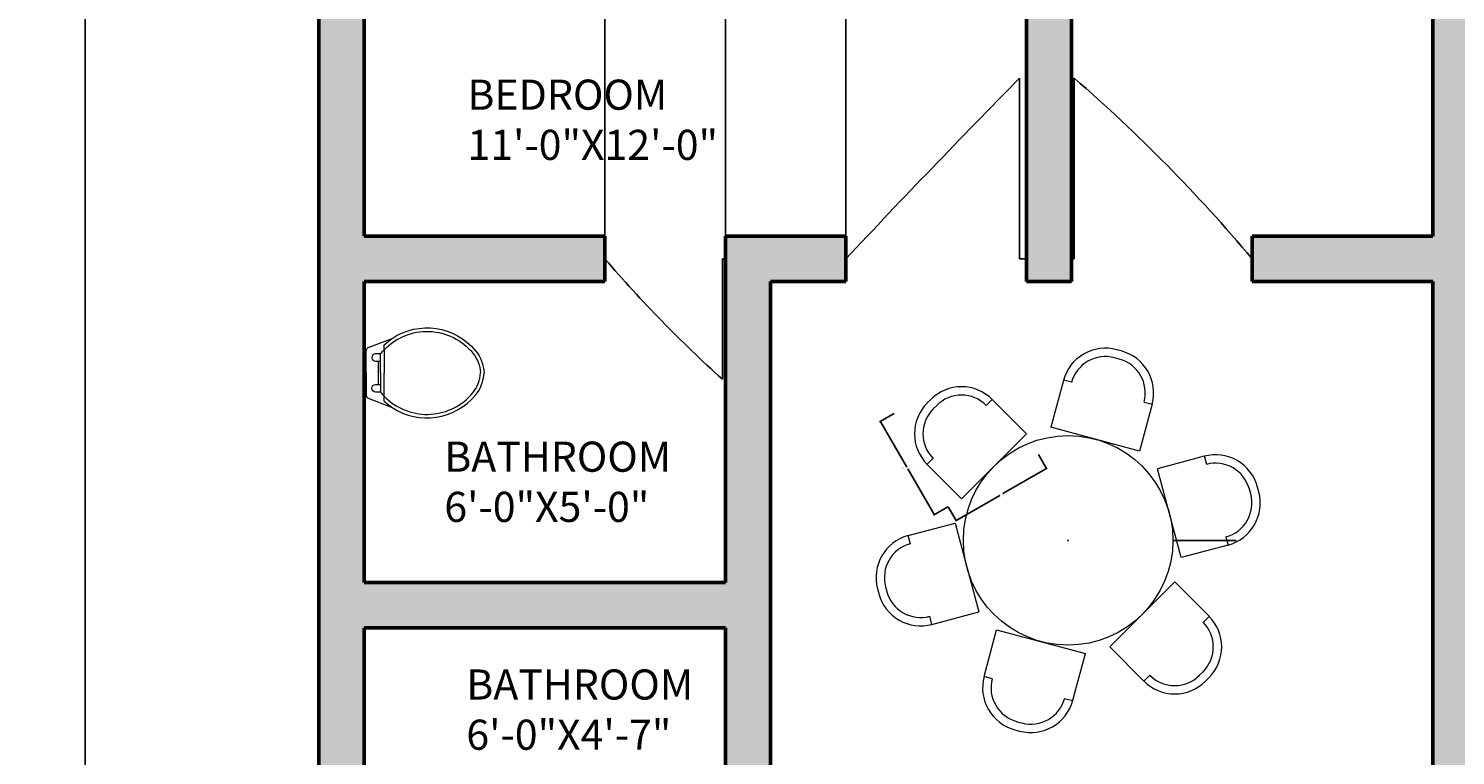
# Model space of a CAD drawing. Units: inches. Extents: x -17 to 536, y -817 to 53.
# Tile 5 of 9: x -17 to 268, y -245 to -100. Entities that reach past the tile are written whole.
import ezdxf

# ---------------------------------------------------------------- set-up
doc = ezdxf.new("R2010")
doc.units = ezdxf.units.IN
doc.header["$MEASUREMENT"] = 0
for name, color, linetype, lineweight in [('A-ANNO-DIMS', 2, 'Continuous', 18), ('A-AREA-IDEN', 7, 'Continuous', 18), ('A-DOOR', 4, 'Continuous', 25), ('A-FLOR-FIXT', 9, 'Continuous', 18), ('A-FURN', 8, 'Continuous', 13), ('A-WALL', 7, 'Continuous', 50), ('A-WALL-PATT', 22, 'Continuous', 13)]:
    doc.layers.add(name, color=color, linetype=linetype, lineweight=lineweight)
doc.styles.get("Standard").update_dxf_attribs({"font": 'arial.ttf'})
doc.dimstyles.get("Standard").update_dxf_attribs({"dimtxt": 0.18, "dimasz": 0.18, "dimexe": 0.18, "dimexo": 0.0625, "dimgap": 0.09, "dimtad": 0, "dimtih": 1, "dimtoh": 1, "dimdec": 0, "dimzin": 0, "dimdsep": 46, "dimlunit": 3, "dimtxsty": 'Standard', "dimcen": 0.09, "dimadec": 0, "dimazin": 0, "dimtfac": 1, "dimtdec": 0, "dimtofl": 0, "dimtmove": 0, "dimatfit": 3, "dimfxl": 1, "dimtolj": 1, "dimtzin": 0, "dimarcsym": 0})

# ---------------------------------------------------------------- blocks, each defined once
blk = doc.blocks.new('*D2')
at = {"layer": 'A-ANNO-DIMS', "color": 0, "lineweight": -2, "transparency": 16777216}
for p, q in [((41.3, 11.55), (-5.38, 11.55)), ((-5.2, 11.37), (-5.2, -378.8)), ((-5.2, -775.27), (-5.2, -385.1)), ((41.3, -775.45), (-5.38, -775.45))]:
    blk.add_line(p, q, dxfattribs=at)
at = {"layer": 'A-ANNO-DIMS', "color": 0, "transparency": 16777216}
for points in [[(-5.23, 11.37), (-5.17, 11.37), (-5.2, 11.55)], [(-5.23, -775.27), (-5.17, -775.27), (-5.2, -775.45)]]:
    blk.add_solid(points, dxfattribs=at)
at = {"layer": 'Defpoints', "color": 0, "transparency": 16777216}
for p in [(41.37, 11.55), (-5.2, -775.45), (41.37, -775.45)]:
    blk.add_point(p, dxfattribs=at)
at = {"layer": 'A-ANNO-DIMS', "color": 0, "transparency": 16777216, "insert": (-5.2, -381.95), "char_height": 6, "attachment_point": 5}
blk.add_mtext('\\A1;65\'-7"', dxfattribs=at)
blk = doc.blocks.new('WC-23IN')
for p, q in [((3.55, 13.58), (3.55, 14.57)), ((3.55, 13.58), (3.55, 8.97)), ((3.55, 4.35), (3.55, 8.97)), ((3.55, 3.36), (3.55, 4.35))]:
    blk.add_line(p, q)
for points in [[(3.55, 13.58, -0.448546), (21.24, 12.93, -0.162618), (22.76, 8.97, -0.470877)], [(5.16, 15.84, -0.383919), (21.78, 13.38, -0.163732), (23.47, 8.97, -0.359733)], [(0, 8.97), (0, 13.45, -0.31031), (0.38, 14), (5.16, 15.84, -0.209071)], [(3.55, 14.57, -0.040937), (5.16, 15.84, -0.163732)], [(2.84, 12.77), (1.86, 12.77, 1), (1.86, 11.28), (2.37, 11.28)], [(2.84, 12.77, -0.022712), (3.55, 13.58, -0.162618)], [(2.84, 8.97), (2.84, 12.77, -0.476108)], [(0, 8.97), (0, 4.48, 0.31031), (0.38, 3.94), (5.16, 2.09, 0.209071)], [(2.84, 8.97), (2.84, 5.16, 0.022712)], [(4.03, 3.88, 0.431639), (21.24, 5, 0.162618), (22.76, 8.97, 0.470877)], [(5.16, 2.09, 0.383919), (21.78, 4.55, 0.163732), (23.47, 8.97, 0.359733)], [(2.84, 5.16), (1.86, 5.16, -1), (1.86, 6.66), (2.37, 6.66)], [(2.84, 5.16, 0.022712), (3.55, 4.35, 0.162618)], [(3.55, 4.35, 0.014165), (4.03, 3.88, 0.162618)], [(3.55, 3.36, 0.040937), (5.16, 2.09, 0.163732)]]:
    blk.add_lwpolyline(points, format="xyb")
for points in [[(2.37, 11.28), (2.37, 6.66)], [(2.37, 11.28), (2.84, 11.28)], [(2.37, 6.66), (2.84, 6.66)]]:
    blk.add_lwpolyline(points)
blk = doc.blocks.new('DINING-CHAIR-STANDARD')
for p, q in [((9.33, 20.2), (0, 17.7)), ((9.85, 18.54), (9.4, 20.21)), ((4.74, 0), (0, 17.7)), ((18.59, 12.68), (18.33, 13.64)), ((20.2, 13.11), (19.94, 14.07)), ((13.64, 4.11), (14.07, 2.5)), ((14.07, 2.5), (4.74, 0))]:
    blk.add_line(p, q)
for centre, radius, start, end in [((11.57, 11.83), 8.66, 15, 105), ((11.57, 11.83), 6.99, 15, 105), ((11.83, 10.87), 6.99, 285, 15), ((11.83, 10.87), 8.66, 285, 15)]:
    blk.add_arc(centre, radius, start, end)
blk = doc.blocks.new('*D14')
at = {"layer": 'A-ANNO-DIMS', "color": 0, "lineweight": -2, "transparency": 16777216}
for p, q in [((155.98, -176.78), (153.09, -178.44)), ((153.34, -178.51), (158.5, -187.45)), ((163.88, -196.76), (158.71, -187.82)), ((166.7, -195.34), (163.81, -197.01))]:
    blk.add_line(p, q, dxfattribs=at)
at = {"layer": 'A-ANNO-DIMS', "color": 0, "transparency": 16777216}
for points in [[(153.37, -178.49), (153.31, -178.52), (153.25, -178.35)], [(163.9, -196.74), (163.85, -196.77), (163.97, -196.92)]]:
    blk.add_solid(points, dxfattribs=at)
at = {"layer": 'Defpoints', "color": 0, "transparency": 16777216}
for p in [(153.25, -178.35), (156.03, -176.75), (166.75, -195.31)]:
    blk.add_point(p, dxfattribs=at)
at = {"layer": 'A-ANNO-DIMS', "color": 0, "transparency": 16777216, "insert": (158.61, -187.63), "char_height": 0.18, "attachment_point": 5}
blk.add_mtext('\\A1;CHAIR A 1\'-9 1/2" TYP.', dxfattribs=at)
blk = doc.blocks.new('*D15')
at = {"layer": 'A-ANNO-DIMS', "color": 0, "lineweight": -2, "transparency": 16777216}
for p, q in [((184.79, -184.97), (186.45, -187.85)), ((186.21, -187.79), (177.67, -192.71)), ((168.51, -198), (177.04, -193.08)), ((166.78, -195.36), (168.45, -198.25))]:
    blk.add_line(p, q, dxfattribs=at)
at = {"layer": 'A-ANNO-DIMS', "color": 0, "transparency": 16777216}
for points in [[(186.19, -187.76), (186.22, -187.81), (186.36, -187.7)], [(168.5, -197.98), (168.53, -198.03), (168.36, -198.09)]]:
    blk.add_solid(points, dxfattribs=at)
at = {"layer": 'Defpoints', "color": 0, "transparency": 16777216}
for p in [(184.75, -184.91), (166.75, -195.31), (168.36, -198.09)]:
    blk.add_point(p, dxfattribs=at)
at = {"layer": 'A-ANNO-DIMS', "color": 0, "transparency": 16777216, "insert": (177.36, -192.89), "char_height": 0.18, "attachment_point": 5}
blk.add_mtext('\\A1;1\'-9" TYP.', dxfattribs=at)
blk = doc.blocks.new('*D41')
at = {"layer": 'A-ANNO-DIMS', "color": 0, "lineweight": -2, "transparency": 16777216}
for p, q in [((98.37, -141.39), (98.37, 53.08)), ((98.55, 52.9), (110.03, 52.9)), ((122.19, 52.9), (110.7, 52.9)), ((122.37, -141.39), (122.37, 53.08))]:
    blk.add_line(p, q, dxfattribs=at)
at = {"layer": 'A-ANNO-DIMS', "color": 0, "transparency": 16777216}
for points in [[(98.55, 52.93), (98.55, 52.87), (98.37, 52.9)], [(122.19, 52.93), (122.19, 52.87), (122.37, 52.9)]]:
    blk.add_solid(points, dxfattribs=at)
at = {"layer": 'Defpoints', "color": 0, "transparency": 16777216}
for p in [(122.37, 52.9), (98.37, -141.45), (122.37, -141.45)]:
    blk.add_point(p, dxfattribs=at)
at = {"layer": 'A-ANNO-DIMS', "color": 0, "transparency": 16777216, "insert": (110.37, 52.9), "char_height": 0.18, "attachment_point": 5}
blk.add_mtext('\\A1;2\'-0"', dxfattribs=at)
blk = doc.blocks.new('*D42')
at = {"layer": 'A-ANNO-DIMS', "color": 0, "lineweight": -2, "transparency": 16777216}
for p, q in [((146.37, -141.39), (146.37, 53.08)), ((146.55, 52.9), (164.04, 52.9)), ((182.19, 52.9), (164.69, 52.9)), ((182.37, -145.89), (182.37, 53.08))]:
    blk.add_line(p, q, dxfattribs=at)
at = {"layer": 'A-ANNO-DIMS', "color": 0, "transparency": 16777216}
for points in [[(146.55, 52.93), (146.55, 52.87), (146.37, 52.9)], [(182.19, 52.93), (182.19, 52.87), (182.37, 52.9)]]:
    blk.add_solid(points, dxfattribs=at)
at = {"layer": 'Defpoints', "color": 0, "transparency": 16777216}
for p in [(182.37, 52.9), (146.37, -141.45), (182.37, -145.95)]:
    blk.add_point(p, dxfattribs=at)
at = {"layer": 'A-ANNO-DIMS', "color": 0, "transparency": 16777216, "insert": (164.37, 52.9), "char_height": 0.18, "attachment_point": 5}
blk.add_mtext('\\A1;3\'-0"', dxfattribs=at)
blk = doc.blocks.new('*D43')
at = {"layer": 'A-ANNO-DIMS', "color": 0, "lineweight": -2, "transparency": 16777216}
for p, q in [((190.58, -202.05), (190.76, -202.05)), ((190.67, -202.14), (190.67, -201.96)), ((224.08, -202.05), (211.73, -202.05))]:
    blk.add_line(p, q, dxfattribs=at)
at = {"layer": 'A-ANNO-DIMS', "color": 0, "transparency": 16777216}
blk.add_solid([(211.73, -202.02), (211.73, -202.08), (211.55, -202.05)], dxfattribs=at)
at = {"layer": 'Defpoints', "color": 0, "transparency": 16777216}
for p in [(169.79, -202.05), (211.55, -202.05)]:
    blk.add_point(p, dxfattribs=at)
at = {"layer": 'A-ANNO-DIMS', "color": 0, "transparency": 16777216, "insert": (224.5, -202.05), "char_height": 0.18, "attachment_point": 5}
blk.add_mtext('\\A1;∅3\'-6"', dxfattribs=at)

msp = doc.modelspace()

# ---------------------------------------------------------------- hatches: boundary and pattern name
at = {"layer": 'A-WALL-PATT'}
h = msp.add_hatch(color=256, dxfattribs=at)
h.dxf.hatch_style = 1
h.paths.add_polyline_path([(217.37, -544.45), (208.37, -544.45), (208.37, -775.45), (217.37, -775.45)], flags=17)
h.paths.add_polyline_path([(327.37, -544.45), (318.37, -544.45), (318.37, -775.45), (327.37, -775.45)], flags=17)
h.paths.add_polyline_path([(494.37, 11.55), (41.37, 11.55), (41.37, -775.45), (50.37, -775.45), (50.37, -739.45), (184.37, -739.45), (184.37, -730.45), (50.37, -730.45), (50.37, -610.45), (172.37, -610.45), (172.37, -601.45), (155.37, -601.45), (155.37, -577.45), (146.37, -577.45), (146.37, -601.45), (50.37, -601.45), (50.37, -553.45), (172.37, -553.45), (172.37, -544.45), (50.37, -544.45), (50.37, -436.45), (191.37, -436.45), (191.37, -319.45), (182.37, -319.45), (182.37, -427.45), (50.37, -427.45), (50.37, -283.45), (98.37, -283.45), (98.37, -274.45), (50.37, -274.45), (50.37, -219.45), (122.37, -219.45), (122.37, -283.45), (191.37, -283.45), (191.37, -274.45), (131.37, -274.45), (131.37, -219.45), (131.37, -150.45), (146.37, -150.45), (146.37, -141.45), (122.37, -141.45), (122.37, -210.45), (50.37, -210.45), (50.37, -150.45), (98.37, -150.45), (98.37, -141.45), (50.37, -141.45), (50.37, 2.55), (182.37, 2.55), (182.37, -150.45), (191.37, -150.45), (191.37, 2.55), (263.37, 2.55), (263.37, -141.45), (227.37, -141.45), (227.37, -150.45), (263.37, -150.45), (263.37, -553.45), (272.37, -553.45), (272.37, -150.45), (308.37, -150.45), (308.37, -141.45), (272.37, -141.45), (272.37, 2.55), (344.37, 2.55), (344.37, -150.45), (353.37, -150.45), (353.37, 2.55), (485.37, 2.55), (485.37, -141.45), (437.37, -141.45), (437.37, -150.45), (485.37, -150.45), (485.37, -210.45), (413.37, -210.45), (413.37, -141.45), (389.37, -141.45), (389.37, -150.45), (404.37, -150.45), (404.37, -219.45), (404.37, -274.45), (353.37, -274.45), (344.37, -274.45), (344.37, -283.45), (353.37, -283.45), (413.37, -283.45), (413.37, -219.45), (485.37, -219.45), (485.37, -274.45), (437.37, -274.45), (437.37, -283.45), (485.37, -283.45), (485.37, -427.45), (353.37, -427.45), (353.37, -319.45), (344.37, -319.45), (344.37, -436.45), (485.37, -436.45), (485.37, -544.45), (363.37, -544.45), (363.37, -553.45), (485.37, -553.45), (485.37, -601.45), (389.37, -601.45), (389.37, -577.45), (380.37, -577.45), (380.37, -601.45), (363.37, -601.45), (363.37, -610.45), (485.37, -610.45), (485.37, -730.45), (351.37, -730.45), (351.37, -739.45), (485.37, -739.45), (485.37, -775.45), (494.37, -775.45)])

# ---------------------------------------------------------------- linework, layer by layer
at = {"layer": 'A-DOOR'}
for p, q in [((180.98, -145.95), (180.98, -109.95)), ((191.87, -145.95), (191.87, -109.95)), ((121.76, -145.95), (122.37, -145.95)), ((121.76, -145.95), (121.76, -169.95)), ((180.98, -145.95), (182.37, -145.95)), ((191.87, -145.95), (191.37, -145.95))]:
    msp.add_line(p, q, dxfattribs=at)
for centre, radius, start, end in [((1840.29, -1739.93), 2325.97, 135.51111, 136.7413), ((-17.85, -352.21), 320.42, 40.0677, 49.1166), ((296.57, 23.86), 261, 220.5881, 227.9509)]:
    msp.add_arc(centre, radius, start, end, dxfattribs=at)
at = {"layer": 'A-FURN'}
msp.add_circle((190.67, -202.05), 20.88, dxfattribs=at)
at = {"layer": 'A-WALL'}
for p, q in [((41.37, 11.55), (41.37, -775.45)), ((50.37, 2.55), (50.37, -141.45)), ((182.37, 2.55), (182.37, -150.45)), ((191.37, 2.55), (191.37, -150.45)), ((263.37, 2.55), (263.37, -141.45)), ((50.37, -141.45), (98.37, -141.45)), ((98.37, -141.45), (98.37, -150.45)), ((122.37, -141.45), (122.37, -210.45)), ((122.37, -141.45), (146.37, -141.45)), ((146.37, -141.45), (146.37, -150.45)), ((227.37, -141.45), (263.37, -141.45)), ((227.37, -141.45), (227.37, -150.45)), ((50.37, -150.45), (98.37, -150.45)), ((50.37, -150.45), (50.37, -210.45)), ((131.37, -150.45), (131.37, -219.45)), ((131.37, -150.45), (146.37, -150.45)), ((182.37, -150.45), (191.37, -150.45)), ((227.37, -150.45), (263.37, -150.45)), ((263.37, -150.45), (263.37, -553.45)), ((50.37, -210.45), (122.37, -210.45)), ((50.37, -219.45), (122.37, -219.45)), ((50.37, -219.45), (50.37, -274.45)), ((122.37, -219.45), (122.37, -283.45)), ((131.37, -219.45), (131.37, -274.45))]:
    msp.add_line(p, q, dxfattribs=at)

# ---------------------------------------------------------------- block references
at = {"layer": 'A-FLOR-FIXT'}
msp.add_blockref('WC-23IN', (50.8, -177.65), dxfattribs=at)
at = {"layer": 'A-FURN'}
for p, rotation in [((202.55, -188.36), 59.99999997356175), ((184.75, -184.91), 120.0000000057707), ((172.87, -198.6), 180), ((196.59, -219.18), 300.0000000082551), ((178.79, -215.74), 239.9999999800936)]:
    msp.add_blockref('DINING-CHAIR-STANDARD', p, dxfattribs=dict(at, rotation=rotation))
msp.add_blockref('DINING-CHAIR-STANDARD', (208.47, -205.49), dxfattribs=at)

# ---------------------------------------------------------------- texts
at = {"layer": 'A-AREA-IDEN', "char_height": 6, "attachment_point": 1}
for s, insert in [('BEDROOM\\P11\'-0"X12\'-0"', (70.96, -110.25)), ('BATHROOM\\P6\'-0"X5\'-0"', (66.35, -182.38)), ('BATHROOM\\P6\'-0"X4\'-7"', (70.74, -227.77))]:
    msp.add_mtext(s, dxfattribs=dict(at, insert=insert))

# ---------------------------------------------------------------- dimensions: what is measured, and where the dimension line sits
at = {"layer": 'A-ANNO-DIMS'}
for base, p1, p2, picture, middle in [((122.37, 52.9), (98.37, -141.45), (122.37, -141.45), '*D41', (110.37, 52.9)), ((182.37, 52.9), (146.37, -141.45), (182.37, -145.95), '*D42', (164.37, 52.9))]:
    dim = msp.add_linear_dim(base=base, p1=p1, p2=p2, dimstyle='Standard', override={"dimdec": 1, "dimlfac": 1, "dimrnd": 0, "dimzin": 1, "dimdsep": 46, "dimlunit": 4, "dimfrac": 2}, dxfattribs=at)
    dim.commit()
    dim.dimension.update_dxf_attribs({"geometry": picture, "text_midpoint": middle})
dim = msp.add_linear_dim(base=(-5.2, -775.45), p1=(41.37, 11.55), p2=(41.37, -775.45), angle=90, dimstyle='Standard', override={"dimtxt": 6, "dimclrd": 0, "dimclre": 0, "dimclrt": 0}, dxfattribs=at)
dim.commit()
dim.dimension.update_dxf_attribs({"geometry": '*D2', "text_midpoint": (-5.2, -381.95)})
for base, p1, p2, angle, text, picture, middle in [((153.25, -178.35), (166.75, -195.31), (156.03, -176.75), 120, 'CHAIR A <> TYP.', '*D14', (158.61, -187.63)), ((168.36, -198.09), (184.75, -184.91), (166.75, -195.31), 210, '<> TYP.', '*D15', (177.36, -192.89))]:
    dim = msp.add_linear_dim(base=base, p1=p1, p2=p2, angle=angle, text=text, dimstyle='Standard', override={"dimdec": 1, "dimlfac": 1, "dimrnd": 0, "dimzin": 1, "dimdsep": 46, "dimlunit": 4, "dimfrac": 2}, dxfattribs=at)
    dim.commit()
    dim.dimension.update_dxf_attribs({"geometry": picture, "text_midpoint": middle})
dim = msp.add_diameter_dim_2p(p1=(169.79, -202.05), p2=(211.55, -202.05), dimstyle='Standard', override={"dimdec": 1, "dimlfac": 1, "dimrnd": 0, "dimzin": 1, "dimdsep": 46, "dimlunit": 4, "dimfrac": 2}, dxfattribs=at)
dim.commit()
dim.dimension.update_dxf_attribs({"geometry": '*D43', "text_midpoint": (224.08, -202.05), "dimtype": 163})

doc.saveas('drawing.dxf')
